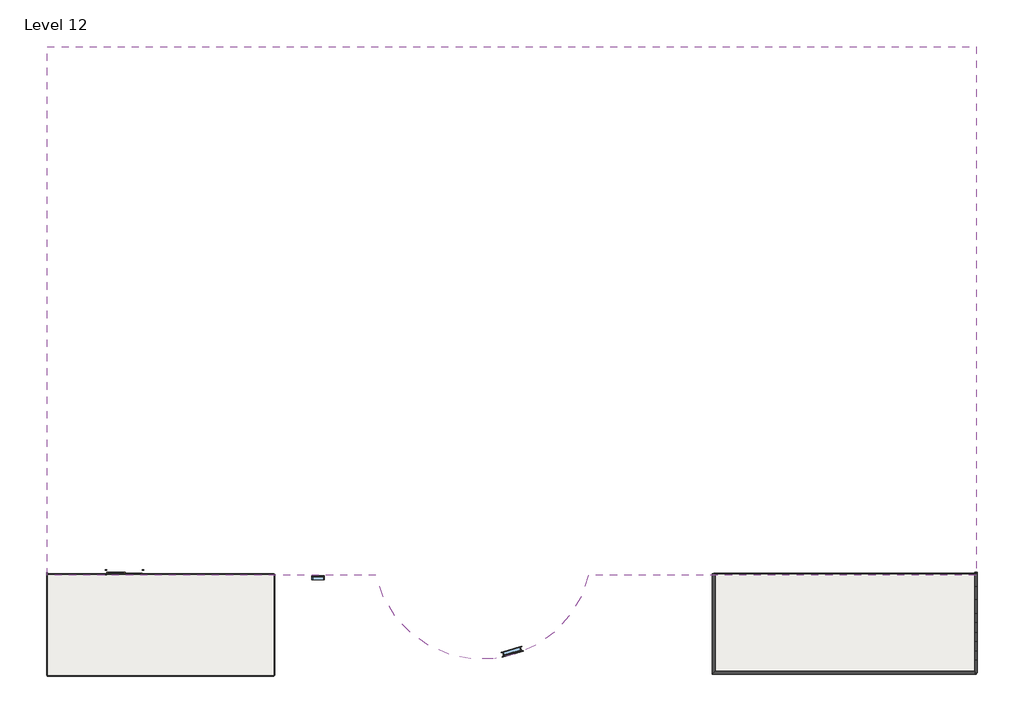
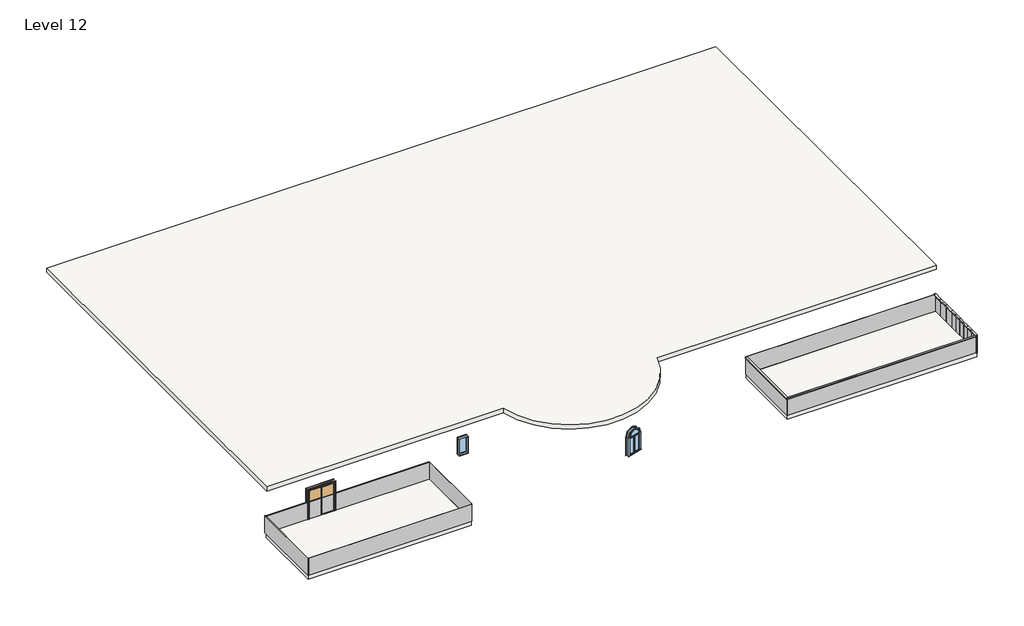
# One storey: 16 plates, 12 members, 3 slabs, 2 windows, 1 door.
"""IFC4 building model written with IfcOpenShell, lengths in millimetres."""

from ifc_helpers import new_model, si_unit, point, frame, frame_2d, origin, place, context, project, spatial, polyline, circle_curve, trimmed, segment, composite_curve, outline, extrude, transform, mapped, element, save
from components import door_076b30e0, member_75074519, member_47bfaf8a, member_9b03179d, member_15823cb3, member_ff8123a6, member_e6b7cb81, system_panel_glazed_cf6986e1, system_panel_glazed_7af1c9c3, system_panel_glazed_a18a7e0a, system_panel_glazed_cc8aff5a, system_panel_glazed_1f2476a4, system_panel_glazed_fe37cdeb, system_panel_glazed_b96adab1, system_panel_glazed_21912a48, system_panel_glazed_a39085c9, window_cf4adaea, window_80bd9af0

model = new_model("IFC4")

# Units and contexts
model_context = context("Model", 3, world=origin())
ifc_project = project(units=[si_unit("LENGTHUNIT", "METRE", prefix="MILLI")], contexts=[model_context])

# Site, building, storey
site = spatial("IfcSite", under=ifc_project)
building = spatial("IfcBuilding", under=site)
storey = spatial("IfcBuildingStorey", under=building, Name="Level 12", Elevation=19812.0)

# Door
placement = place(None, origin())
door_shape = door_076b30e0(model_context)
element("IfcDoor", 1, ObjectType="Door-Double-Sliding : 68\" x 80\"", at=placement, inside=storey, context=model_context, shape_type="MappedRepresentation", body=[
    mapped(door_shape, transform((-16064.585279, -12227.7237084, 19812.0), x_axis=(-1.0, 0.0, 0.0), y_axis=(0.0, -1.0, 0.0), z_axis=(0.0, 0.0, 1.0))),
])

# Members
member_shape = member_75074519(model_context)
element("IfcMember", 2, ObjectType="Rectangular Mullion : 2.5\" x 5\" rectangular", at=placement, inside=storey, context=model_context, shape_type="MappedRepresentation", body=[
    mapped(member_shape, transform((25489.814721, -17253.9328285, 21031.2), x_axis=(1.0, 0.0, 0.0), y_axis=(0.0, 1.0, 0.0), z_axis=(0.0, 0.0, 1.0))),
])
member_2_shape = member_47bfaf8a(model_context)
element("IfcMember", 3, ObjectType="Rectangular Mullion : 2.5\" x 5\" rectangular", at=placement, inside=storey, context=model_context, shape_type="MappedRepresentation", body=[
    mapped(member_2_shape, transform((25489.814721, -17253.9328285, 21031.2), x_axis=(0.0, 0.0, 1.0), y_axis=(-1.0, 0.0, 0.0), z_axis=(0.0, -1.0, 0.0))),
])
member_3_shape = member_9b03179d(model_context)
element("IfcMember", 4, ObjectType="Rectangular Mullion : 2.5\" x 5\" rectangular", at=placement, inside=storey, context=model_context, shape_type="MappedRepresentation", body=[
    mapped(member_3_shape, transform((25489.814721, -13022.5934151, 21031.2), x_axis=(0.0, 0.0, 1.0), y_axis=(-1.0, 0.0, 0.0), z_axis=(0.0, -1.0, 0.0))),
])
element("IfcMember", 5, ObjectType="Rectangular Mullion : 2.5\" x 5\" rectangular", at=placement, inside=storey, context=model_context, shape_type="MappedRepresentation", body=[
    mapped(member_3_shape, transform((25489.814721, -13690.4631218, 21031.2), x_axis=(0.0, 0.0, 1.0), y_axis=(-1.0, 0.0, 0.0), z_axis=(0.0, -1.0, 0.0))),
])
element("IfcMember", 6, ObjectType="Rectangular Mullion : 2.5\" x 5\" rectangular", at=placement, inside=storey, context=model_context, shape_type="MappedRepresentation", body=[
    mapped(member_3_shape, transform((25489.814721, -14358.3328285, 21031.2), x_axis=(0.0, 0.0, 1.0), y_axis=(-1.0, 0.0, 0.0), z_axis=(0.0, -1.0, 0.0))),
])
member_4_shape = member_15823cb3(model_context)
element("IfcMember", 7, ObjectType="Rectangular Mullion : 2.5\" x 5\" rectangular", at=placement, inside=storey, context=model_context, shape_type="MappedRepresentation", body=[
    mapped(member_4_shape, transform((25489.814721, -14815.5328285, 21031.2), x_axis=(0.0, 0.0, 1.0), y_axis=(-1.0, 0.0, 0.0), z_axis=(0.0, -1.0, 0.0))),
])
element("IfcMember", 8, ObjectType="Rectangular Mullion : 2.5\" x 5\" rectangular", at=placement, inside=storey, context=model_context, shape_type="MappedRepresentation", body=[
    mapped(member_4_shape, transform((25489.814721, -15272.7328285, 21031.2), x_axis=(0.0, 0.0, 1.0), y_axis=(-1.0, 0.0, 0.0), z_axis=(0.0, -1.0, 0.0))),
])
element("IfcMember", 9, ObjectType="Rectangular Mullion : 2.5\" x 5\" rectangular", at=placement, inside=storey, context=model_context, shape_type="MappedRepresentation", body=[
    mapped(member_4_shape, transform((25489.814721, -15729.9328285, 21031.2), x_axis=(0.0, 0.0, 1.0), y_axis=(-1.0, 0.0, 0.0), z_axis=(0.0, -1.0, 0.0))),
])
element("IfcMember", 10, ObjectType="Rectangular Mullion : 2.5\" x 5\" rectangular", at=placement, inside=storey, context=model_context, shape_type="MappedRepresentation", body=[
    mapped(member_4_shape, transform((25489.814721, -16187.1328285, 21031.2), x_axis=(0.0, 0.0, 1.0), y_axis=(-1.0, 0.0, 0.0), z_axis=(0.0, -1.0, 0.0))),
])
element("IfcMember", 11, ObjectType="Rectangular Mullion : 2.5\" x 5\" rectangular", at=placement, inside=storey, context=model_context, shape_type="MappedRepresentation", body=[
    mapped(member_4_shape, transform((25489.814721, -16644.3328285, 21031.2), x_axis=(0.0, 0.0, 1.0), y_axis=(-1.0, 0.0, 0.0), z_axis=(0.0, -1.0, 0.0))),
])
member_5_shape = member_ff8123a6(model_context)
element("IfcMember", 12, ObjectType="Rectangular Mullion : 2.5\" x 5\" rectangular", at=placement, inside=storey, context=model_context, shape_type="MappedRepresentation", body=[
    mapped(member_5_shape, transform((12685.8483935, -12432.2309773, 21031.2), x_axis=(0.0, 0.0, 1.0), y_axis=(1.0, 0.0, 0.0), z_axis=(0.0, 1.0, 0.0))),
])
member_6_shape = member_e6b7cb81(model_context)
element("IfcMember", 13, ObjectType="Rectangular Mullion : 2.5\" x 5\" rectangular", at=placement, inside=storey, context=model_context, shape_type="MappedRepresentation", body=[
    mapped(member_6_shape, transform((12685.8483935, -17253.9328285, 21031.2), x_axis=(0.0, 0.0, 1.0), y_axis=(0.0, 1.0, 0.0), z_axis=(-1.0, 0.0, 0.0))),
])

# Plates
system_panel_glazed_shape = system_panel_glazed_cf6986e1(model_context)
element("IfcPlate", 14, ObjectType="System Panel : Glazed", at=placement, inside=storey, context=model_context, shape_type="MappedRepresentation", body=[
    mapped(system_panel_glazed_shape, transform((19087.8315572, -12432.2309773, 19812.0), x_axis=(1.0, 0.0, 0.0), y_axis=(0.0, 1.0, 0.0), z_axis=(0.0, 0.0, 1.0))),
])
system_panel_glazed_2_shape = system_panel_glazed_7af1c9c3(model_context)
element("IfcPlate", 15, ObjectType="System Panel : Glazed", at=placement, inside=storey, context=model_context, shape_type="MappedRepresentation", body=[
    mapped(system_panel_glazed_2_shape, transform((25489.814721, -16949.1328285, 19812.0), x_axis=(0.0, -1.0, 0.0), y_axis=(1.0, 0.0, 0.0), z_axis=(0.0, 0.0, 1.0))),
])
system_panel_glazed_3_shape = system_panel_glazed_a18a7e0a(model_context)
element("IfcPlate", 16, ObjectType="System Panel : Glazed", at=placement, inside=storey, context=model_context, shape_type="MappedRepresentation", body=[
    mapped(system_panel_glazed_3_shape, transform((25489.814721, -16415.7328285, 19812.0), x_axis=(0.0, -1.0, 0.0), y_axis=(1.0, 0.0, 0.0), z_axis=(0.0, 0.0, 1.0))),
])
element("IfcPlate", 17, ObjectType="System Panel : Glazed", at=placement, inside=storey, context=model_context, shape_type="MappedRepresentation", body=[
    mapped(system_panel_glazed_3_shape, transform((25489.814721, -15958.5328285, 19812.0), x_axis=(0.0, -1.0, 0.0), y_axis=(1.0, 0.0, 0.0), z_axis=(0.0, 0.0, 1.0))),
])
element("IfcPlate", 18, ObjectType="System Panel : Glazed", at=placement, inside=storey, context=model_context, shape_type="MappedRepresentation", body=[
    mapped(system_panel_glazed_3_shape, transform((25489.814721, -15501.3328285, 19812.0), x_axis=(0.0, -1.0, 0.0), y_axis=(1.0, 0.0, 0.0), z_axis=(0.0, 0.0, 1.0))),
])
element("IfcPlate", 19, ObjectType="System Panel : Glazed", at=placement, inside=storey, context=model_context, shape_type="MappedRepresentation", body=[
    mapped(system_panel_glazed_3_shape, transform((25489.814721, -15044.1328285, 19812.0), x_axis=(0.0, -1.0, 0.0), y_axis=(1.0, 0.0, 0.0), z_axis=(0.0, 0.0, 1.0))),
])
element("IfcPlate", 20, ObjectType="System Panel : Glazed", at=placement, inside=storey, context=model_context, shape_type="MappedRepresentation", body=[
    mapped(system_panel_glazed_3_shape, transform((25489.814721, -14586.9328285, 19812.0), x_axis=(0.0, -1.0, 0.0), y_axis=(1.0, 0.0, 0.0), z_axis=(0.0, 0.0, 1.0))),
])
system_panel_glazed_4_shape = system_panel_glazed_cc8aff5a(model_context)
element("IfcPlate", 21, ObjectType="System Panel : Glazed", at=placement, inside=storey, context=model_context, shape_type="MappedRepresentation", body=[
    mapped(system_panel_glazed_4_shape, transform((25489.814721, -12688.6585617, 19812.0), x_axis=(0.0, -1.0, 0.0), y_axis=(1.0, 0.0, 0.0), z_axis=(0.0, 0.0, 1.0))),
])
element("IfcPlate", 22, ObjectType="System Panel : Glazed", at=placement, inside=storey, context=model_context, shape_type="MappedRepresentation", body=[
    mapped(system_panel_glazed_4_shape, transform((25489.814721, -14024.3979752, 19812.0), x_axis=(0.0, -1.0, 0.0), y_axis=(1.0, 0.0, 0.0), z_axis=(0.0, 0.0, 1.0))),
])
element("IfcPlate", 23, ObjectType="System Panel : Glazed", at=placement, inside=storey, context=model_context, shape_type="MappedRepresentation", body=[
    mapped(system_panel_glazed_4_shape, transform((25489.814721, -13356.5282684, 19812.0), x_axis=(0.0, -1.0, 0.0), y_axis=(1.0, 0.0, 0.0), z_axis=(0.0, 0.0, 1.0))),
])
system_panel_glazed_5_shape = system_panel_glazed_1f2476a4(model_context)
element("IfcPlate", 24, ObjectType="System Panel : Glazed", at=placement, inside=storey, context=model_context, shape_type="MappedRepresentation", body=[
    mapped(system_panel_glazed_5_shape, transform((19056.0815572, -17253.9328285, 19812.0), x_axis=(-1.0, 0.0, 0.0), y_axis=(0.0, -1.0, 0.0), z_axis=(0.0, 0.0, 1.0))),
])
system_panel_glazed_6_shape = system_panel_glazed_fe37cdeb(model_context)
element("IfcPlate", 25, ObjectType="System Panel : Glazed", at=placement, inside=storey, context=model_context, shape_type="MappedRepresentation", body=[
    mapped(system_panel_glazed_6_shape, transform((12685.8483935, -14843.0819029, 19812.0), x_axis=(0.0, 1.0, 0.0), y_axis=(-1.0, 0.0, 0.0), z_axis=(0.0, 0.0, 1.0))),
])
system_panel_glazed_7_shape = system_panel_glazed_b96adab1(model_context)
element("IfcPlate", 26, ObjectType="System Panel : Glazed", at=placement, inside=storey, context=model_context, shape_type="MappedRepresentation", body=[
    mapped(system_panel_glazed_7_shape, transform((-14302.7926538, -12456.3237084, 19812.0), x_axis=(1.0, 0.0, 0.0), y_axis=(0.0, 1.0, 0.0), z_axis=(0.0, 0.0, 1.0))),
])
element("IfcPlate", 27, ObjectType="System Panel : Glazed", at=placement, inside=storey, context=model_context, shape_type="MappedRepresentation", body=[
    mapped(system_panel_glazed_7_shape, transform((-14302.7926538, -17381.2674651, 19812.0), x_axis=(-1.0, 0.0, 0.0), y_axis=(0.0, -1.0, 0.0), z_axis=(0.0, 0.0, 1.0))),
])
system_panel_glazed_8_shape = system_panel_glazed_21912a48(model_context)
element("IfcPlate", 28, ObjectType="System Panel : Glazed", at=placement, inside=storey, context=model_context, shape_type="MappedRepresentation", body=[
    mapped(system_panel_glazed_8_shape, transform((-8781.8000285, -14918.7955867, 19812.0), x_axis=(0.0, -1.0, 0.0), y_axis=(1.0, 0.0, 0.0), z_axis=(0.0, 0.0, 1.0))),
])
system_panel_glazed_9_shape = system_panel_glazed_a39085c9(model_context)
element("IfcPlate", 29, ObjectType="System Panel : Glazed", at=placement, inside=storey, context=model_context, shape_type="MappedRepresentation", body=[
    mapped(system_panel_glazed_9_shape, transform((-19823.785279, -14867.9955867, 19812.0), x_axis=(0.0, 1.0, 0.0), y_axis=(-1.0, 0.0, 0.0), z_axis=(0.0, 0.0, 1.0))),
])

# Slabs
element("IfcSlab", 30, ObjectType="Generic - 12\"", at=placement, inside=storey, context=model_context, shape_type="SweptSolid", body=[
    extrude(outline(composite_curve([segment(polyline([(25489.814721, 13301.2686816), (25489.814721, -12505.1313184), (6571.5594464, -12505.1313184)]), True, "CONTINUOUS"), segment(trimmed(circle_curve(frame_2d((1385.214721, -11274.4982772)), 5330.3498284), [point((6571.5594464, -12505.1313184))], [point((-3801.1300045, -12505.1313184))], False, "CARTESIAN"), True, "CONTINUOUS"), segment(polyline([(-3801.1300045, -12505.1313184), (-19823.785279, -12505.1313184), (-19823.785279, 13301.2686816), (25489.814721, 13301.2686816)]), True, "CONTINUOUS")], self_intersect=False)), frame((0.0, 0.0, 22859.5903029), z_axis=(0.0, 0.0, 1.0), x_axis=(1.0, 0.0, 0.0)), (0.0, 0.0, 1.0), 304.8),
])
element("IfcSlab", 31, ObjectType="Generic - 12\"", at=placement, inside=storey, context=model_context, shape_type="SweptSolid", body=[
    extrude(outline(polyline([(25489.814721, -12431.9741109), (25489.814721, -17253.9328285), (12688.8765791, -17253.9328285), (12688.8765791, -12431.9741109), (25489.814721, -12431.9741109)])), frame((0.0, 0.0, 19507.2), z_axis=(0.0, 0.0, 1.0), x_axis=(1.0, 0.0, 0.0)), (0.0, 0.0, 1.0), 304.8),
])
element("IfcSlab", 32, ObjectType="Generic - 12\"", at=placement, inside=storey, context=model_context, shape_type="SweptSolid", body=[
    extrude(outline(polyline([(-8781.8000285, -12456.3237084), (-8781.8000285, -17381.2674651), (-19823.785279, -17381.2674651), (-19823.785279, -12456.3237084), (-8781.8000285, -12456.3237084)])), frame((0.0, 0.0, 19507.2), z_axis=(0.0, 0.0, 1.0), x_axis=(1.0, 0.0, 0.0)), (0.0, 0.0, 1.0), 304.8),
])

# Windows
window_shape = window_cf4adaea(model_context)
element("IfcWindow", 33, ObjectType="36\" x 48\"", at=placement, inside=storey, context=model_context, shape_type="MappedRepresentation", body=[
    mapped(window_shape, transform((2854.4373201, -16223.3134577, 19057.1107236), x_axis=(-0.9598322746039031, -0.2805744190561527, 0.0), y_axis=(0.2805744190561527, -0.9598322746039031, 0.0), z_axis=(0.0, 0.0, 1.0))),
])
window_2_shape = window_80bd9af0(model_context)
element("IfcWindow", 34, ObjectType="Fixed : 24\" x 48\"", at=placement, inside=storey, context=model_context, shape_type="MappedRepresentation", body=[
    mapped(window_2_shape, transform((-6577.685279, -12617.2007309, 20064.613139), x_axis=(1.0, 0.0, 0.0), y_axis=(0.0, 1.0, 0.0), z_axis=(0.0, 0.0, 1.0))),
])

save(model, "model.ifc")

# Revit data of these elements
# Type "Door-Double-Sliding : 68\" x 80\""
#   Type Mark = "10"
#   Construction Type Id = "opn-d45"
#   Assembly Code = "C1020"
#   Analytic Construction = "Wood frame, double glass door "
#   Thickness = 0' - 2"
#   Thermal Resistance (R) = 1.8150 (h·ft²·°F)/BTU
#   Heat Transfer Coefficient (U) = 0.5510 BTU/(h·ft²·°F)
#   Height = 6' - 8"
#   Rail Width = 0' - 2"
#   Stiles = 0' - 2"
#   Trim Projection Ext = 0' - 1"
#   Trim Projection Int = 0' - 1"
#   Trim Width = 0' - 3"
#   Width = 5' - 8"
#   Define Thermal Properties by = 1
#   Glazing = Glass
#   Panel Material = Wood - Birch - Solid Stained Light Low Gloss
#   Trim Material = Paint - Sienna
#   Visual Light Transmittance = 0
#   Solar Heat Gain Coefficient = 0
#   Function = (empty or 0)
#   Wall Closure = (empty or 0)
# Type "Rectangular Mullion : 2.5\" x 5\" rectangular"
#   built-in parameter 1007304 = 0.416667 (stored number, unit not read)
#   built-in parameter 1007301 = 0.104167 (stored number, unit not read)
#   built-in parameter 1007300 = 0.104167 (stored number, unit not read)
# Type "System Panel : Glazed"
#   Construction Type Id = "GSP4R"
#   Analytic Construction = "1/8 in Pilkington single glazing"
#   Visual Light Transmittance = 0.9
#   Solar Heat Gain Coefficient = 0.86
#   Heat Transfer Coefficient (U) = 1.18115 BTU/(h·ft²·°F)
# Type "Generic - 12\""
#   Assembly Code = "B1010"
#   Function = 0
#   Layers, outside or top first: 1' - 0" no material (function 1)
# Type "36\" x 48\""
#   Type Mark = "38"
#   Construction Type Id = "SGL"
#   Assembly Code = "B2020100"
#   Analytic Construction = "Large single-glazed windows"
#   Visual Light Transmittance = 0.9
#   Solar Heat Gain Coefficient = 0.86
#   Heat Transfer Coefficient (U) = 0.979472 BTU/(h·ft²·°F)
#   Height = 4' - 0"
#   Default Sill Height = 3' - 0"
#   Trim Projection - Ext. = 0' - 0 1/2"
#   Trim Projection - Int. = 0' - 0 3/4"
#   Trim Width - Exterior = 0' - 3 1/2"
#   Trim Width - Interior = 0' - 3 1/2"
#   Width = 3' - 0"
#   Window Inset = 0' - 0 3/4"
#   Define Thermal Properties by = 1
#   Glass Pane Material = Glass
#   Sash Material = Sash
#   Trim Exterior Material = Trim
#   Trim Interior Material = Trim
#   Wall Closure = (empty or 0)
# Type "Fixed : 24\" x 48\""
#   Type Mark = "2"
#   Construction Type Id = "GSP4R"
#   Assembly Code = "B2020100"
#   Analytic Construction = "1/8 in Pilkington single glazing"
#   Visual Light Transmittance = 0.9
#   Solar Heat Gain Coefficient = 0.78
#   Heat Transfer Coefficient (U) = 0.6496 BTU/(h·ft²·°F)
#   Height = 4' - 0"
#   Default Sill Height = 3' - 0"
#   Width = 2' - 0"
#   Window Inset = 0' - 0 3/4"
#   Define Thermal Properties by = 1
#   Glass Pane Material = Glass
#   Sash Material = Sash
#   Wall Closure = (empty or 0)
# Element 1 (IfcDoor, "Door-Double-Sliding : 68\" x 80\"")
#   Phase Created = New Construction
#   Materials on its faces: "Paint - Sienna", "Wood - Birch - Solid Stained Light Low Gloss", "Glass"
# Elements 2, 3, 4, 5, 6, 7, 8, 9, 10, 11, 12, 13 (IfcMember, "Rectangular Mullion : 2.5\" x 5\" rectangular")
#   Phase Created = New Construction
#   Materials on its faces: "Aluminum"
# Elements 14, 15, 16, 17, 18, 19, 20, 21, 22, 23, 24, 25, 26, 27, 28, 29 (IfcPlate, "System Panel : Glazed")
#   Phase Created = New Construction
#   Materials on its faces: "Glass"
# Element 30 (IfcSlab, "Generic - 12\"")
#   Height Offset From Level = 10' - 11.98387"
#   Phase Created = New Construction
#   Materials on its faces: "Default Floor"
# Elements 31, 32 (IfcSlab, "Generic - 12\"")
#   Height Offset From Level = 0' - 0"
#   Phase Created = New Construction
#   Materials on its faces: "Default Floor"
# Element 33 (IfcWindow, "36\" x 48\"")
#   Mark = "28"
#   Phase Created = New Construction
#   Materials on its faces: "Sash", "Trim", "Glass"
# Element 34 (IfcWindow, "Fixed : 24\" x 48\"")
#   Mark = "79"
#   Phase Created = New Construction
#   Materials on its faces: "Sash", "Glass"
# Materials
#   "Glass": class "Glass", colour RGB 0 128 192, transparency 0.75, Description = "Soda Lime Glass", Cost = 0
#   "Wood - Birch - Solid Stained Light Low Gloss": class "Wood", colour RGB 210 159 95, transparency 0, Cost = 0
#   "Paint - Sienna": colour RGB 118 70 51, transparency 0, Cost = 0
#   "Sash": class "Wood", colour RGB 224 178 126, transparency 0
#   "Trim": class "Wood", colour RGB 224 178 126, transparency 0
#   "Aluminum": class "Metal", colour RGB 247 247 247, transparency 0, Description = "Aluminum 6061", Cost = 0
#   "Default Floor": colour RGB 128 128 128, transparency 0
